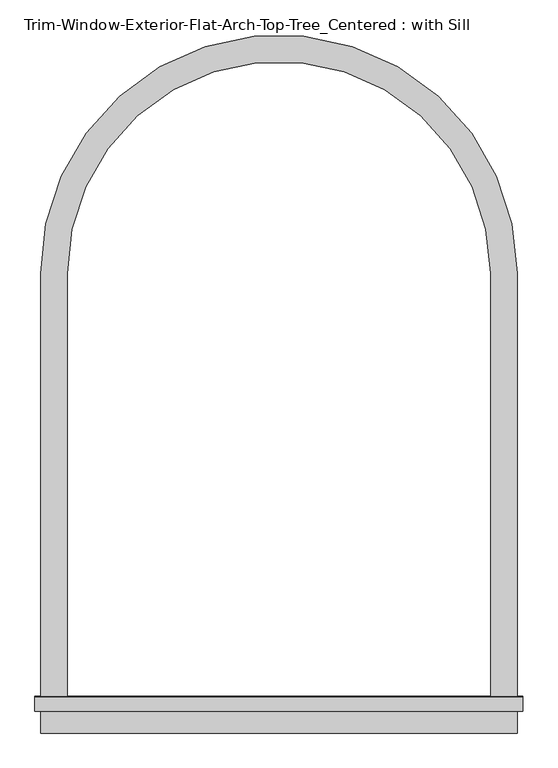
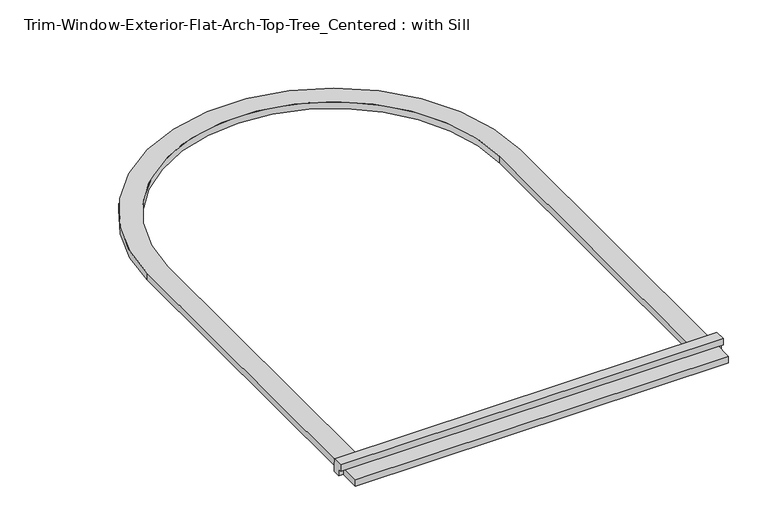
"""IFC4 building model written with IfcOpenShell, lengths in millimetres: proxy geometry, Trim-Window-Exterior-Flat-Arch-Top-Tree_Centered : with Sill."""

from ifc_helpers import new_model, si_unit, point, frame, frame_2d, origin, origin_with_axes, place, context, project, spatial, polyline, circle_curve, trimmed, segment, composite_curve, outline, extrude, source, transform, mapped, element, save


def trim_window_exterior_flat_arch_top_tree_centered_with_sill_aed3e54d(model_context):
    return source(origin(), model_context, "Body", "SweptSolid", [
        extrude(outline(polyline([(514.35, -1393.7823709), (514.35, -1450.9323709), (-514.35, -1450.9323709), (-514.35, -1393.7823709), (514.35, -1393.7823709)])), origin_with_axes(), (0.0, 0.0, 1.0), 19.05),
        extrude(outline(polyline([(-1403.35, 38.1), (-1374.0580645, 38.1), (-1371.6, 19.05), (-1371.6, 0.0), (-1393.7823709, 0.0), (-1393.7823709, 19.05), (-1403.35, 19.05), (-1403.35, 38.1)])), frame((-527.05, 0.0, 0.0), z_axis=(1.0, 0.0, 0.0), x_axis=(0.0, 1.0, 0.0)), (0.0, 0.0, 1.0), 1054.1),
        extrude(outline(composite_curve([segment(trimmed(circle_curve(frame_2d((0.0, -457.2)), 514.35), [point((-514.35, -457.2))], [point((514.35, -457.2))], False, "CARTESIAN"), True, "CONTINUOUS"), segment(polyline([(514.35, -457.2), (514.35, -1371.6), (457.2, -1371.6), (457.2, -457.2)]), True, "CONTINUOUS"), segment(trimmed(circle_curve(frame_2d((0.0, -457.2)), 457.2), [point((457.2, -457.2))], [point((-457.2, -457.2))], True, "CARTESIAN"), True, "CONTINUOUS"), segment(polyline([(-457.2, -457.2), (-457.2, -1371.6), (-514.35, -1371.6), (-514.35, -457.2)]), True, "CONTINUOUS")], self_intersect=False)), origin_with_axes(), (0.0, 0.0, 1.0), 19.05),
    ])


if __name__ == "__main__":
    model = new_model("IFC4")
    model_context = context("Model", 3, world=origin())
    ifc_project = project(units=[si_unit("LENGTHUNIT", "METRE", prefix="MILLI")], contexts=[model_context])
    site = spatial("IfcSite", under=ifc_project)
    building = spatial("IfcBuilding", under=site)
    placement = place(None, origin())
    trim_window_exterior_flat_arch_top_tree_centered_with_sill_shape = trim_window_exterior_flat_arch_top_tree_centered_with_sill_aed3e54d(model_context)
    element("IfcBuildingElementProxy", 1, Name="Trim-Window-Exterior-Flat-Arch-Top-Tree_Centered : with Sill", ObjectType="Trim-Window-Exterior-Flat-Arch-Top-Tree_Centered : with Sill", at=placement, inside=building, context=model_context, shape_type="MappedRepresentation", body=[
        mapped(trim_window_exterior_flat_arch_top_tree_centered_with_sill_shape, transform((0.0, 0.0, 0.0), x_axis=(1.0, 0.0, 0.0), y_axis=(0.0, 1.0, 0.0), z_axis=(0.0, 0.0, 1.0))),
    ])
    save(model, "model.ifc")

# Revit data of these elements
# Type "Trim-Window-Exterior-Flat-Arch-Top-Tree_Centered : with Sill"
#   Trim Width = 0' - 2 1/4"
#   Trim Thickness_Picture Frame = 0' - 1 1/4"
#   Trim Thickness_with Sill = 0' - 0 3/4"
#   Sill Thickness = 0' - 1 1/4"
#   Opening Width [instance default] = 2' - 0"
#   Opening Height [instance default] = 3' - 0"
#   Default Elevation = 4' - 0"
#   Sill = yes
#   Picture Frame = no
#   Trim Material [instance default] = none
# Element 1 (IfcBuildingElementProxy, "Trim-Window-Exterior-Flat-Arch-Top-Tree_Centered : with Sill")
#   Opening Width = 3' - 0"
#   Opening Height = 4' - 6"
#   Trim Material = Clad - White
#   Materials on its faces: "Clad - White"
# Materials
#   "Clad - White": class "Wood", colour RGB 242 242 238, transparency 0, Cost = 0
